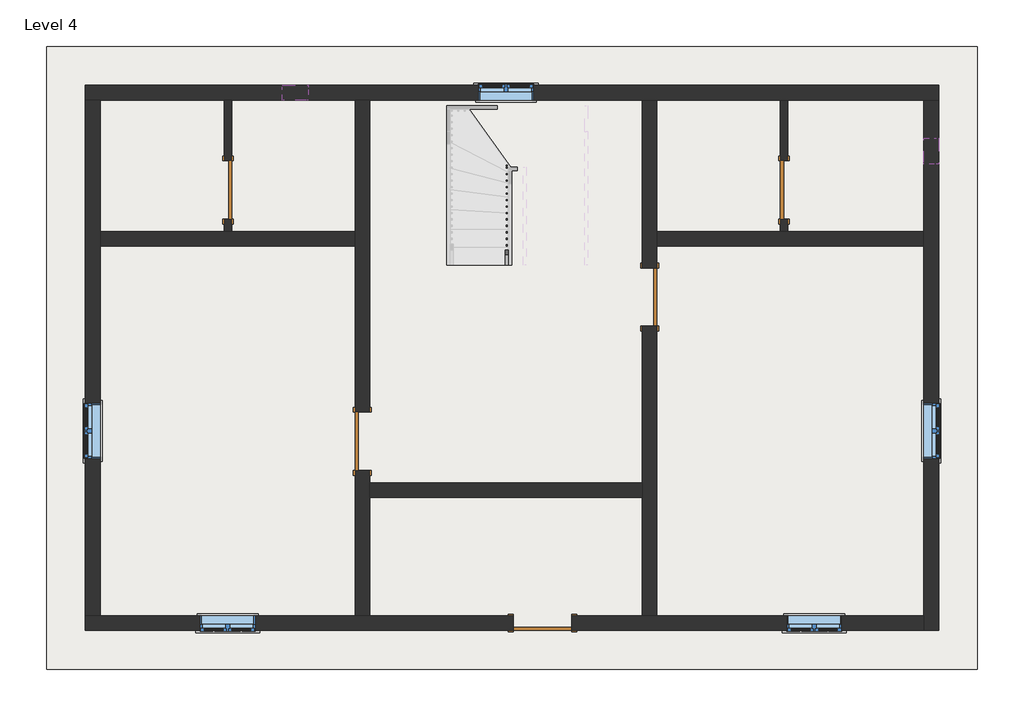
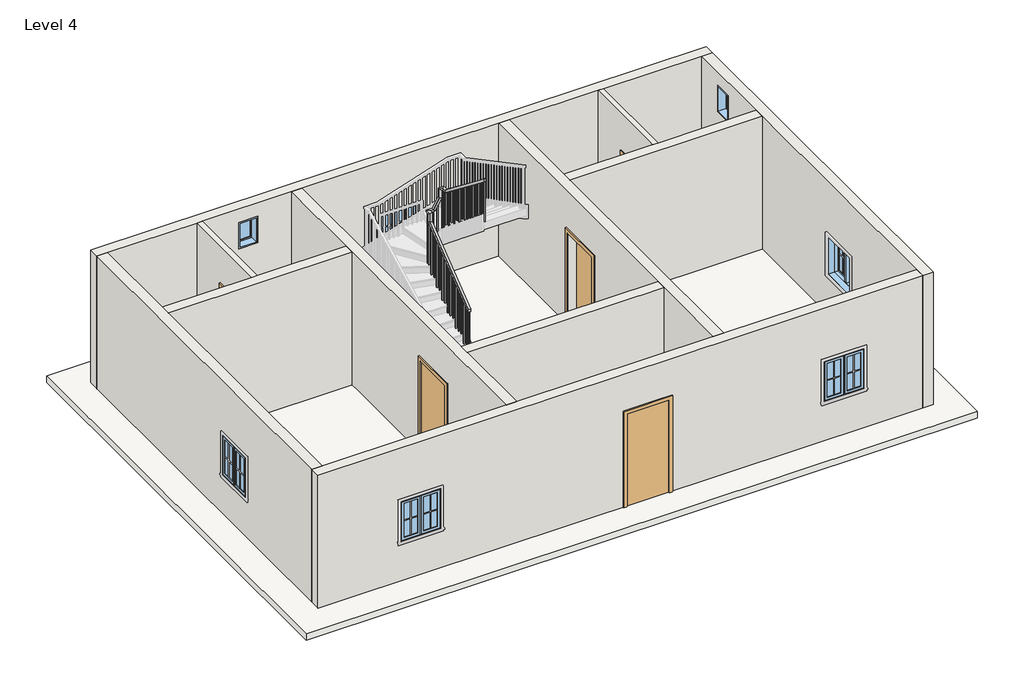
# One storey, part 1 of 2: 11 walls, 7 windows, 5 doors, 1 railing, 1 roof.
"""IFC4 building model written with IfcOpenShell, lengths in millimetres."""

from ifc_helpers import new_model, si_unit, frame, origin, place, context, project, spatial, polyline, outline, extrude, faceted_brep, transform, mapped, element, save
from components import door_e5f9f3c4, door_a90ba1ad, door_305aa2a5, door_0ca8825f, window_aa618e30, window_339605e1

model = new_model("IFC4")

# Units and contexts
model_context = context("Model", 3, world=origin())
ifc_project = project(units=[si_unit("LENGTHUNIT", "METRE", prefix="MILLI")], contexts=[model_context])

# Site, building, storey
site = spatial("IfcSite", under=ifc_project)
building = spatial("IfcBuilding", under=site)
storey = spatial("IfcBuildingStorey", under=building, Name="Level 4", Elevation=6400.8)

# Doors
placement = place(None, origin())
door_shape = door_e5f9f3c4(model_context)
element("IfcDoor", 1, ObjectType="Single-Flush : 36\" x 84\"", at=placement, inside=storey, context=model_context, shape_type="MappedRepresentation", body=[
    mapped(door_shape, transform((-5102.9390964, 4820.103532, 6400.8), x_axis=(0.0, -1.0, 0.0), y_axis=(1.0, 0.0, 0.0), z_axis=(0.0, 0.0, 1.0))),
])
door_2_shape = door_a90ba1ad(model_context)
element("IfcDoor", 2, ObjectType="Single-Flush : 36\" x 84\"", at=placement, inside=storey, context=model_context, shape_type="MappedRepresentation", body=[
    mapped(door_2_shape, transform((-3001.0890964, 883.103532, 6400.8), x_axis=(0.0, -1.0, 0.0), y_axis=(1.0, 0.0, 0.0), z_axis=(0.0, 0.0, 1.0))),
])
element("IfcDoor", 3, ObjectType="Single-Flush : 36\" x 84\"", at=placement, inside=storey, context=model_context, shape_type="MappedRepresentation", body=[
    mapped(door_2_shape, transform((1494.7109036, 3143.703532, 6400.8), x_axis=(0.0, 1.0, 0.0), y_axis=(-1.0, 0.0, 0.0), z_axis=(0.0, 0.0, 1.0))),
])
door_3_shape = door_305aa2a5(model_context)
element("IfcDoor", 4, ObjectType="Single-Flush : 36\" x 84\"", at=placement, inside=storey, context=model_context, shape_type="MappedRepresentation", body=[
    mapped(door_3_shape, transform((3596.5609036, 4820.103532, 6400.8), x_axis=(0.0, -1.0, 0.0), y_axis=(1.0, 0.0, 0.0), z_axis=(0.0, 0.0, 1.0))),
])
door_4_shape = door_0ca8825f(model_context)
element("IfcDoor", 5, ObjectType="Single-Flush : 36\" x 84\"", at=placement, inside=storey, context=model_context, shape_type="MappedRepresentation", body=[
    mapped(door_4_shape, transform((-181.6890964, -1961.696468, 6400.8), x_axis=(-1.0, 0.0, 0.0), y_axis=(0.0, -1.0, 0.0), z_axis=(0.0, 0.0, 1.0))),
])

# Railing
element("IfcRailing", 6, ObjectType="Handrail - Rectangular", at=placement, inside=storey, context=model_context, shape_type="SolidModel", body=[
    faceted_brep([(-765.8890964, 3647.9718401, 7484.5333333), (-765.8890964, 3647.9718401, 7420.2000346), (-715.0890964, 3647.9718401, 7420.2000346), (-715.0890964, 3647.9718401, 7484.5333333), (-765.8890964, 5099.503532, 8612.4191036), (-765.8890964, 5150.303532, 8587.5590024), (-715.0890964, 5150.303532, 8587.5590024), (-715.0890964, 5099.503532, 8612.4191036), (-765.8890964, 5099.503532, 8815.4281882), (-765.8890964, 5150.303532, 8764.6281882), (-715.0890964, 5150.303532, 8764.6281882), (-715.0890964, 5099.503532, 8815.4281882), (-765.8890964, 5226.503532, 8815.4281882), (-765.8890964, 5226.503532, 8764.6281882), (-715.0890964, 5175.703532, 8764.6281882), (-715.0890964, 5175.703532, 8815.4281882), (-638.8890964, 5226.503532, 8815.4281882), (-609.7677625, 5226.503532, 8764.6281882), (-609.7677625, 5175.703532, 8764.6281882), (-638.8890964, 5175.703532, 8815.4281882), (-511.8890964, 5226.503532, 9032.3051451), (-461.0890964, 5226.503532, 9018.5256424), (-461.0890964, 5175.703532, 9018.5256424), (-511.8890964, 5175.703532, 9032.3051451), (-511.8890964, 5226.503532, 9235.3142297), (-461.0890964, 5226.503532, 9184.5142297), (-461.0890964, 5175.703532, 9184.5142297), (-511.8890964, 5175.703532, 9235.3142297), (-384.8890964, 5226.503532, 9235.3142297), (-384.8890964, 5226.503532, 9184.5142297), (-435.6890964, 5175.703532, 9184.5142297), (-435.6890964, 5175.703532, 9235.3142297), (-384.8890964, 5099.503532, 9235.3142297), (-384.8890964, 5082.086864, 9184.5142297), (-435.6890964, 5082.086864, 9184.5142297), (-435.6890964, 5099.503532, 9235.3142297), (-384.8890964, 3647.9718401, 10363.2), (-435.6890964, 3647.9718401, 10363.2), (-435.6890964, 3647.9718401, 10298.8667013), (-384.8890964, 3647.9718401, 10298.8667013)], [[[0, 1, 2, 3]], [[1, 0, 4, 5]], [[2, 1, 5, 6]], [[3, 2, 6, 7]], [[0, 3, 7, 4]], [[5, 4, 8, 9]], [[6, 5, 9, 10]], [[7, 6, 10, 11]], [[4, 7, 11, 8]], [[9, 8, 12, 13]], [[10, 9, 13, 14]], [[11, 10, 14, 15]], [[8, 11, 15, 12]], [[13, 12, 16, 17]], [[14, 13, 17, 18]], [[15, 14, 18, 19]], [[12, 15, 19, 16]], [[17, 16, 20, 21]], [[18, 17, 21, 22]], [[19, 18, 22, 23]], [[16, 19, 23, 20]], [[21, 20, 24, 25]], [[22, 21, 25, 26]], [[23, 22, 26, 27]], [[20, 23, 27, 24]], [[25, 24, 28, 29]], [[26, 25, 29, 30]], [[27, 26, 30, 31]], [[24, 27, 31, 28]], [[29, 28, 32, 33]], [[30, 29, 33, 34]], [[31, 30, 34, 35]], [[28, 31, 35, 32]], [[36, 37, 38, 39]], [[33, 32, 36, 39]], [[34, 33, 39, 38]], [[35, 34, 38, 37]], [[32, 35, 37, 36]]]),
    extrude(outline(polyline([(3667.578532, 10283.6316852), (3686.628532, 10268.8292361), (3686.628532, 9279.4666667), (3667.578532, 9279.4666667), (3667.578532, 10283.6316852)])), frame((-419.8140964, 0.0, 0.0), z_axis=(1.0, 0.0, 0.0), x_axis=(0.0, 1.0, 0.0)), (0.0, 0.0, 1.0), 19.05),
    extrude(outline(polyline([(3769.178532, 10204.6852902), (3788.228532, 10189.8828411), (3788.228532, 9279.4666667), (3769.178532, 9279.4666667), (3769.178532, 10204.6852902)])), frame((-419.8140964, 0.0, 0.0), z_axis=(1.0, 0.0, 0.0), x_axis=(0.0, 1.0, 0.0)), (0.0, 0.0, 1.0), 19.05),
    extrude(outline(polyline([(3870.778532, 10125.7388952), (3889.828532, 10110.9364462), (3889.828532, 9279.4666667), (3870.778532, 9279.4666667), (3870.778532, 10125.7388952)])), frame((-419.8140964, 0.0, 0.0), z_axis=(1.0, 0.0, 0.0), x_axis=(0.0, 1.0, 0.0)), (0.0, 0.0, 1.0), 19.05),
    extrude(outline(polyline([(3972.378532, 10046.7925003), (3991.428532, 10031.9900512), (3991.428532, 9110.1333333), (3972.378532, 9110.1333333), (3972.378532, 10046.7925003)])), frame((-419.8140964, 0.0, 0.0), z_axis=(1.0, 0.0, 0.0), x_axis=(0.0, 1.0, 0.0)), (0.0, 0.0, 1.0), 19.05),
    extrude(outline(polyline([(4073.978532, 9967.8461053), (4093.028532, 9953.0436562), (4093.028532, 9110.1333333), (4073.978532, 9110.1333333), (4073.978532, 9967.8461053)])), frame((-419.8140964, 0.0, 0.0), z_axis=(1.0, 0.0, 0.0), x_axis=(0.0, 1.0, 0.0)), (0.0, 0.0, 1.0), 19.05),
    extrude(outline(polyline([(4175.578532, 9888.8997103), (4194.628532, 9874.0972613), (4194.628532, 9110.1333333), (4175.578532, 9110.1333333), (4175.578532, 9888.8997103)])), frame((-419.8140964, 0.0, 0.0), z_axis=(1.0, 0.0, 0.0), x_axis=(0.0, 1.0, 0.0)), (0.0, 0.0, 1.0), 19.05),
    extrude(outline(polyline([(4277.178532, 9809.9533154), (4296.228532, 9795.1508663), (4296.228532, 8940.8), (4277.178532, 8940.8), (4277.178532, 9809.9533154)])), frame((-419.8140964, 0.0, 0.0), z_axis=(1.0, 0.0, 0.0), x_axis=(0.0, 1.0, 0.0)), (0.0, 0.0, 1.0), 19.05),
    extrude(outline(polyline([(4378.778532, 9731.0069204), (4397.828532, 9716.2044713), (4397.828532, 8940.8), (4378.778532, 8940.8), (4378.778532, 9731.0069204)])), frame((-419.8140964, 0.0, 0.0), z_axis=(1.0, 0.0, 0.0), x_axis=(0.0, 1.0, 0.0)), (0.0, 0.0, 1.0), 19.05),
    extrude(outline(polyline([(4480.378532, 9652.0605254), (4499.428532, 9637.2580764), (4499.428532, 8771.4666667), (4480.378532, 8771.4666667), (4480.378532, 9652.0605254)])), frame((-419.8140964, 0.0, 0.0), z_axis=(1.0, 0.0, 0.0), x_axis=(0.0, 1.0, 0.0)), (0.0, 0.0, 1.0), 19.05),
    extrude(outline(polyline([(4581.978532, 9573.1141304), (4601.028532, 9558.3116814), (4601.028532, 8771.4666667), (4581.978532, 8771.4666667), (4581.978532, 9573.1141304)])), frame((-419.8140964, 0.0, 0.0), z_axis=(1.0, 0.0, 0.0), x_axis=(0.0, 1.0, 0.0)), (0.0, 0.0, 1.0), 19.05),
    extrude(outline(polyline([(4683.578532, 9494.1677355), (4702.628532, 9479.3652864), (4702.628532, 8771.4666667), (4683.578532, 8771.4666667), (4683.578532, 9494.1677355)])), frame((-419.8140964, 0.0, 0.0), z_axis=(1.0, 0.0, 0.0), x_axis=(0.0, 1.0, 0.0)), (0.0, 0.0, 1.0), 19.05),
    extrude(outline(polyline([(4785.178532, 9415.2213405), (4804.228532, 9400.4188914), (4804.228532, 8602.1333333), (4785.178532, 8602.1333333), (4785.178532, 9415.2213405)])), frame((-419.8140964, 0.0, 0.0), z_axis=(1.0, 0.0, 0.0), x_axis=(0.0, 1.0, 0.0)), (0.0, 0.0, 1.0), 19.05),
    extrude(outline(polyline([(4886.778532, 9336.2749455), (4905.828532, 9321.4724965), (4905.828532, 8602.1333333), (4886.778532, 8602.1333333), (4886.778532, 9336.2749455)])), frame((-419.8140964, 0.0, 0.0), z_axis=(1.0, 0.0, 0.0), x_axis=(0.0, 1.0, 0.0)), (0.0, 0.0, 1.0), 19.05),
    extrude(outline(polyline([(4988.378532, 9257.3285506), (5007.428532, 9242.5261015), (5007.428532, 8432.8), (4988.378532, 8432.8), (4988.378532, 9257.3285506)])), frame((-419.8140964, 0.0, 0.0), z_axis=(1.0, 0.0, 0.0), x_axis=(0.0, 1.0, 0.0)), (0.0, 0.0, 1.0), 19.05),
    extrude(outline(polyline([(5089.978532, 9178.3821556), (5109.028532, 9163.5797065), (5109.028532, 8432.8), (5089.978532, 8432.8), (5089.978532, 9178.3821556)])), frame((-419.8140964, 0.0, 0.0), z_axis=(1.0, 0.0, 0.0), x_axis=(0.0, 1.0, 0.0)), (0.0, 0.0, 1.0), 19.05),
    extrude(outline(polyline([(-445.2140964, 5191.578532), (-445.2140964, 5210.628532), (-426.1640964, 5210.628532), (-426.1640964, 5191.578532), (-445.2140964, 5191.578532)])), frame((0.0, 0.0, 8094.1333333), z_axis=(0.0, 0.0, 1.0), x_axis=(1.0, 0.0, 0.0)), (0.0, 0.0, 1.0), 1090.3808964),
    extrude(outline(polyline([(8904.66524, -527.7640964), (8872.1336964, -546.8140964), (7924.8, -546.8140964), (7924.8, -527.7640964), (8904.66524, -527.7640964)])), frame((0.0, 5191.578532, 0.0), z_axis=(0.0, 1.0, 0.0), x_axis=(0.0, 0.0, 1.0)), (0.0, 0.0, 1.0), 19.05),
    extrude(outline(polyline([(8731.1636744, -629.3640964), (8698.6321309, -648.4140964), (7755.4666667, -648.4140964), (7755.4666667, -629.3640964), (8731.1636744, -629.3640964)])), frame((0.0, 5191.578532, 0.0), z_axis=(0.0, 1.0, 0.0), x_axis=(0.0, 0.0, 1.0)), (0.0, 0.0, 1.0), 19.05),
    extrude(outline(polyline([(-730.9640964, 5162.4468401), (-750.0140964, 5162.4468401), (-750.0140964, 5181.4968401), (-730.9640964, 5181.4968401), (-730.9640964, 5162.4468401)])), frame((0.0, 0.0, 7586.1333333), z_axis=(0.0, 0.0, 1.0), x_axis=(1.0, 0.0, 0.0)), (0.0, 0.0, 1.0), 1178.4948549),
    extrude(outline(polyline([(5060.8468401, 8518.0483397), (5079.8968401, 8532.8507888), (5079.8968401, 7416.8), (5060.8468401, 7416.8), (5060.8468401, 8518.0483397)])), frame((-750.0140964, 0.0, 0.0), z_axis=(1.0, 0.0, 0.0), x_axis=(0.0, 1.0, 0.0)), (0.0, 0.0, 1.0), 19.05),
    extrude(outline(polyline([(4959.2468401, 8439.1019447), (4978.2968401, 8453.9043938), (4978.2968401, 7416.8), (4959.2468401, 7416.8), (4959.2468401, 8439.1019447)])), frame((-750.0140964, 0.0, 0.0), z_axis=(1.0, 0.0, 0.0), x_axis=(0.0, 1.0, 0.0)), (0.0, 0.0, 1.0), 19.05),
    extrude(outline(polyline([(4857.6468401, 8360.1555498), (4876.6968401, 8374.9579988), (4876.6968401, 7247.4666667), (4857.6468401, 7247.4666667), (4857.6468401, 8360.1555498)])), frame((-750.0140964, 0.0, 0.0), z_axis=(1.0, 0.0, 0.0), x_axis=(0.0, 1.0, 0.0)), (0.0, 0.0, 1.0), 19.05),
    extrude(outline(polyline([(4756.0468401, 8281.2091548), (4775.0968401, 8296.0116039), (4775.0968401, 7247.4666667), (4756.0468401, 7247.4666667), (4756.0468401, 8281.2091548)])), frame((-750.0140964, 0.0, 0.0), z_axis=(1.0, 0.0, 0.0), x_axis=(0.0, 1.0, 0.0)), (0.0, 0.0, 1.0), 19.05),
    extrude(outline(polyline([(4654.4468401, 8202.2627598), (4673.4968401, 8217.0652089), (4673.4968401, 7078.1333333), (4654.4468401, 7078.1333333), (4654.4468401, 8202.2627598)])), frame((-750.0140964, 0.0, 0.0), z_axis=(1.0, 0.0, 0.0), x_axis=(0.0, 1.0, 0.0)), (0.0, 0.0, 1.0), 19.05),
    extrude(outline(polyline([(4552.8468401, 8123.3163649), (4571.8968401, 8138.1188139), (4571.8968401, 7078.1333333), (4552.8468401, 7078.1333333), (4552.8468401, 8123.3163649)])), frame((-750.0140964, 0.0, 0.0), z_axis=(1.0, 0.0, 0.0), x_axis=(0.0, 1.0, 0.0)), (0.0, 0.0, 1.0), 19.05),
    extrude(outline(polyline([(4451.2468401, 8044.3699699), (4470.2968401, 8059.1724189), (4470.2968401, 6908.8), (4451.2468401, 6908.8), (4451.2468401, 8044.3699699)])), frame((-750.0140964, 0.0, 0.0), z_axis=(1.0, 0.0, 0.0), x_axis=(0.0, 1.0, 0.0)), (0.0, 0.0, 1.0), 19.05),
    extrude(outline(polyline([(4349.6468401, 7965.4235749), (4368.6968401, 7980.226024), (4368.6968401, 6908.8), (4349.6468401, 6908.8), (4349.6468401, 7965.4235749)])), frame((-750.0140964, 0.0, 0.0), z_axis=(1.0, 0.0, 0.0), x_axis=(0.0, 1.0, 0.0)), (0.0, 0.0, 1.0), 19.05),
    extrude(outline(polyline([(4248.0468401, 7886.4771799), (4267.0968401, 7901.279629), (4267.0968401, 6908.8), (4248.0468401, 6908.8), (4248.0468401, 7886.4771799)])), frame((-750.0140964, 0.0, 0.0), z_axis=(1.0, 0.0, 0.0), x_axis=(0.0, 1.0, 0.0)), (0.0, 0.0, 1.0), 19.05),
    extrude(outline(polyline([(4146.4468401, 7807.530785), (4165.4968401, 7822.333234), (4165.4968401, 6739.4666667), (4146.4468401, 6739.4666667), (4146.4468401, 7807.530785)])), frame((-750.0140964, 0.0, 0.0), z_axis=(1.0, 0.0, 0.0), x_axis=(0.0, 1.0, 0.0)), (0.0, 0.0, 1.0), 19.05),
    extrude(outline(polyline([(4044.8468401, 7728.58439), (4063.8968401, 7743.3868391), (4063.8968401, 6739.4666667), (4044.8468401, 6739.4666667), (4044.8468401, 7728.58439)])), frame((-750.0140964, 0.0, 0.0), z_axis=(1.0, 0.0, 0.0), x_axis=(0.0, 1.0, 0.0)), (0.0, 0.0, 1.0), 19.05),
    extrude(outline(polyline([(3943.2468401, 7649.637995), (3962.2968401, 7664.4404441), (3962.2968401, 6739.4666667), (3943.2468401, 6739.4666667), (3943.2468401, 7649.637995)])), frame((-750.0140964, 0.0, 0.0), z_axis=(1.0, 0.0, 0.0), x_axis=(0.0, 1.0, 0.0)), (0.0, 0.0, 1.0), 19.05),
    extrude(outline(polyline([(3841.6468401, 7570.6916001), (3860.6968401, 7585.4940491), (3860.6968401, 6570.1333333), (3841.6468401, 6570.1333333), (3841.6468401, 7570.6916001)])), frame((-750.0140964, 0.0, 0.0), z_axis=(1.0, 0.0, 0.0), x_axis=(0.0, 1.0, 0.0)), (0.0, 0.0, 1.0), 19.05),
    extrude(outline(polyline([(3740.0468401, 7491.7452051), (3759.0968401, 7506.5476541), (3759.0968401, 6570.1333333), (3740.0468401, 6570.1333333), (3740.0468401, 7491.7452051)])), frame((-750.0140964, 0.0, 0.0), z_axis=(1.0, 0.0, 0.0), x_axis=(0.0, 1.0, 0.0)), (0.0, 0.0, 1.0), 19.05),
    extrude(outline(polyline([(-419.8140964, 5191.578532), (-419.8140964, 5210.628532), (-400.7640964, 5210.628532), (-400.7640964, 5191.578532), (-419.8140964, 5191.578532)])), frame((0.0, 0.0, 8263.4666667), z_axis=(0.0, 0.0, 1.0), x_axis=(1.0, 0.0, 0.0)), (0.0, 0.0, 1.0), 921.0475631),
    extrude(outline(polyline([(-730.9640964, 5191.578532), (-750.0140964, 5191.578532), (-750.0140964, 5210.628532), (-730.9640964, 5210.628532), (-730.9640964, 5191.578532)])), frame((0.0, 0.0, 7586.1333333), z_axis=(0.0, 0.0, 1.0), x_axis=(1.0, 0.0, 0.0)), (0.0, 0.0, 1.0), 1178.4948549),
    extrude(outline(polyline([(3647.9718401, 10298.8667013), (3667.0218401, 10284.0642523), (3667.0218401, 9279.4666667), (3647.9718401, 9279.4666667), (3647.9718401, 10298.8667013)])), frame((-419.8140964, 0.0, 0.0), z_axis=(1.0, 0.0, 0.0), x_axis=(0.0, 1.0, 0.0)), (0.0, 0.0, 1.0), 19.05),
    extrude(outline(polyline([(3647.9718401, 7420.2000346), (3667.0218401, 7435.0024837), (3667.0218401, 6570.1333333), (3647.9718401, 6570.1333333), (3647.9718401, 7420.2000346)])), frame((-750.0140964, 0.0, 0.0), z_axis=(1.0, 0.0, 0.0), x_axis=(0.0, 1.0, 0.0)), (0.0, 0.0, 1.0), 19.05),
])

# Roof
element("IfcRoof", 7, ObjectType="Generic - 12\"", at=placement, inside=storey, context=model_context, shape_type="SweptSolid", body=[
    extrude(outline(polyline([(-7944.5640964, 7068.003532), (6625.5109036, 7068.003532), (6625.5109036, -2685.596468), (-7944.5640964, -2685.596468), (-7944.5640964, 7068.003532)])), frame((0.0, 0.0, 6248.4), z_axis=(0.0, 0.0, 1.0), x_axis=(1.0, 0.0, 0.0)), (0.0, 0.0, 1.0), 152.4),
])

# Walls
element("IfcWall", 8, ObjectType="WALL4.5\"", at=placement, inside=storey, context=model_context, shape_type="SweptSolid", body=[
    extrude(outline(polyline([(4362.903532, 8534.4), (4362.903532, 6400.8), (4172.403532, 6400.8), (4172.403532, 9448.8), (6229.803532, 9448.8), (6229.803532, 6400.8), (5277.303532, 6400.8), (5277.303532, 8534.4), (4362.903532, 8534.4)])), frame((-5160.0890964, 0.0, 0.0), z_axis=(1.0, 0.0, 0.0), x_axis=(0.0, 1.0, 0.0)), (0.0, 0.0, 1.0), 114.3),
])
element("IfcWall", 9, ObjectType="WALL4.5\"", at=placement, inside=storey, context=model_context, shape_type="SweptSolid", body=[
    extrude(outline(polyline([(4362.903532, 8534.4), (4362.903532, 6400.8), (4172.403532, 6400.8), (4172.403532, 9448.8), (6229.803532, 9448.8), (6229.803532, 6400.8), (5277.303532, 6400.8), (5277.303532, 8534.4), (4362.903532, 8534.4)])), frame((3539.4109036, 0.0, 0.0), z_axis=(1.0, 0.0, 0.0), x_axis=(0.0, 1.0, 0.0)), (0.0, 0.0, 1.0), 114.3),
])
element("IfcWall", 10, ObjectType="WALL9\"", at=placement, inside=storey, context=model_context, shape_type="Brep", body=[
    faceted_brep([(-7334.9640964, 6229.803532, 6400.8), (-7106.3640964, 6229.803532, 6400.8), (-5160.0890964, 6229.803532, 6400.8), (-5045.7890964, 6229.803532, 6400.8), (-3115.3890964, 6229.803532, 6400.8), (-2886.7890964, 6229.803532, 6400.8), (1380.4109036, 6229.803532, 6400.8), (1609.0109036, 6229.803532, 6400.8), (3539.4109036, 6229.803532, 6400.8), (3653.7109036, 6229.803532, 6400.8), (5787.3109036, 6229.803532, 6400.8), (6015.9109036, 6229.803532, 6400.8), (6015.9109036, 6229.803532, 9448.8), (5787.3109036, 6229.803532, 9448.8), (3653.7109036, 6229.803532, 9448.8), (3539.4109036, 6229.803532, 9448.8), (1609.0109036, 6229.803532, 9448.8), (1380.4109036, 6229.803532, 9448.8), (-2886.7890964, 6229.803532, 9448.8), (-3115.3890964, 6229.803532, 9448.8), (-5045.7890964, 6229.803532, 9448.8), (-5160.0890964, 6229.803532, 9448.8), (-7106.3640964, 6229.803532, 9448.8), (-7334.9640964, 6229.803532, 9448.8), (-3848.8140964, 6229.803532, 9144.0), (-3848.8140964, 6229.803532, 8534.4), (-4255.2140964, 6229.803532, 8534.4), (-4255.2140964, 6229.803532, 9144.0), (-321.3890964, 6229.803532, 8229.6), (-321.3890964, 6229.803532, 7315.2), (-1184.9890964, 6229.803532, 7315.2), (-1184.9890964, 6229.803532, 8229.6), (-7334.9640964, 6458.403532, 6400.8), (-7334.9640964, 6458.403532, 9448.8), (6015.9109036, 6458.403532, 9448.8), (6015.9109036, 6458.403532, 6400.8), (-3848.8140964, 6458.403532, 9144.0), (-4255.2140964, 6458.403532, 9144.0), (-4255.2140964, 6458.403532, 8534.4), (-3848.8140964, 6458.403532, 8534.4), (-321.3890964, 6458.403532, 8229.6), (-1184.9890964, 6458.403532, 8229.6), (-1184.9890964, 6458.403532, 7315.2), (-321.3890964, 6458.403532, 7315.2)], [[[0, 1, 2, 3, 4, 5, 6, 7, 8, 9, 10, 11, 12, 13, 14, 15, 16, 17, 18, 19, 20, 21, 22, 23], [24, 25, 26, 27], [28, 29, 30, 31]], [[32, 33, 34, 35], [36, 37, 38, 39], [40, 41, 42, 43]], [[11, 10, 9, 8, 7, 6, 5, 4, 3, 2, 1, 0, 32, 35]], [[12, 11, 35, 34]], [[0, 23, 33, 32]], [[25, 24, 36, 39]], [[26, 25, 39, 38]], [[27, 26, 38, 37]], [[24, 27, 37, 36]], [[29, 28, 40, 43]], [[30, 29, 43, 42]], [[31, 30, 42, 41]], [[28, 31, 41, 40]], [[23, 22, 21, 20, 19, 18, 17, 16, 15, 14, 13, 12, 34, 33]]]),
])
element("IfcWall", 11, ObjectType="WALL9\"", at=placement, inside=storey, context=model_context, shape_type="Brep", body=[
    faceted_brep([(5787.3109036, 6229.803532, 6400.8), (5787.3109036, 4172.403532, 6400.8), (5787.3109036, 3943.803532, 6400.8), (5787.3109036, -1847.396468, 6400.8), (5787.3109036, -2075.996468, 6400.8), (5787.3109036, -2075.996468, 9448.8), (5787.3109036, -1847.396468, 9448.8), (5787.3109036, 3943.803532, 9448.8), (5787.3109036, 4172.403532, 9448.8), (5787.3109036, 6229.803532, 9448.8), (5787.3109036, 5226.503532, 9144.0), (5787.3109036, 5226.503532, 8534.4), (5787.3109036, 5632.903532, 8534.4), (5787.3109036, 5632.903532, 9144.0), (5787.3109036, 616.403532, 8229.6), (5787.3109036, 616.403532, 7315.2), (5787.3109036, 1480.003532, 7315.2), (5787.3109036, 1480.003532, 8229.6), (6015.9109036, 6229.803532, 6400.8), (6015.9109036, 6229.803532, 9448.8), (6015.9109036, -2075.996468, 9448.8), (6015.9109036, -2075.996468, 6400.8), (6015.9109036, 5226.503532, 9144.0), (6015.9109036, 5632.903532, 9144.0), (6015.9109036, 5632.903532, 8534.4), (6015.9109036, 5226.503532, 8534.4), (6015.9109036, 616.403532, 8229.6), (6015.9109036, 1480.003532, 8229.6), (6015.9109036, 1480.003532, 7315.2), (6015.9109036, 616.403532, 7315.2)], [[[0, 1, 2, 3, 4, 5, 6, 7, 8, 9], [10, 11, 12, 13], [14, 15, 16, 17]], [[18, 19, 20, 21], [22, 23, 24, 25], [26, 27, 28, 29]], [[4, 3, 2, 1, 0, 18, 21]], [[0, 9, 19, 18]], [[5, 4, 21, 20]], [[11, 10, 22, 25]], [[12, 11, 25, 24]], [[13, 12, 24, 23]], [[10, 13, 23, 22]], [[15, 14, 26, 29]], [[16, 15, 29, 28]], [[17, 16, 28, 27]], [[14, 17, 27, 26]], [[9, 8, 7, 6, 5, 20, 19]]]),
])
element("IfcWall", 12, ObjectType="WALL9\"", at=placement, inside=storey, context=model_context, shape_type="Brep", body=[
    faceted_brep([(-638.8890964, -1847.396468, 8534.4), (-638.8890964, -1847.396468, 6400.8), (-2886.7890964, -1847.396468, 6400.8), (-3115.3890964, -1847.396468, 6400.8), (-7106.3640964, -1847.396468, 6400.8), (-7334.9640964, -1847.396468, 6400.8), (-7334.9640964, -1847.396468, 9448.8), (-7106.3640964, -1847.396468, 9448.8), (-3115.3890964, -1847.396468, 9448.8), (-2886.7890964, -1847.396468, 9448.8), (1380.4109036, -1847.396468, 9448.8), (1609.0109036, -1847.396468, 9448.8), (5787.3109036, -1847.396468, 9448.8), (5787.3109036, -1847.396468, 6400.8), (1609.0109036, -1847.396468, 6400.8), (1380.4109036, -1847.396468, 6400.8), (275.5109036, -1847.396468, 6400.8), (275.5109036, -1847.396468, 8534.4), (-5542.6765964, -1847.396468, 8229.6), (-5542.6765964, -1847.396468, 7315.2), (-4679.0765964, -1847.396468, 7315.2), (-4679.0765964, -1847.396468, 8229.6), (3641.0109036, -1847.396468, 8229.6), (3641.0109036, -1847.396468, 7315.2), (4504.6109036, -1847.396468, 7315.2), (4504.6109036, -1847.396468, 8229.6), (-7334.9640964, -2075.996468, 6400.8), (-638.8890964, -2075.996468, 6400.8), (-638.8890964, -2075.996468, 8534.4), (275.5109036, -2075.996468, 8534.4), (275.5109036, -2075.996468, 6400.8), (5787.3109036, -2075.996468, 6400.8), (5787.3109036, -2075.996468, 9448.8), (-7334.9640964, -2075.996468, 9448.8), (-5542.6765964, -2075.996468, 8229.6), (-4679.0765964, -2075.996468, 8229.6), (-4679.0765964, -2075.996468, 7315.2), (-5542.6765964, -2075.996468, 7315.2), (3641.0109036, -2075.996468, 8229.6), (4504.6109036, -2075.996468, 8229.6), (4504.6109036, -2075.996468, 7315.2), (3641.0109036, -2075.996468, 7315.2)], [[[0, 1, 2, 3, 4, 5, 6, 7, 8, 9, 10, 11, 12, 13, 14, 15, 16, 17], [18, 19, 20, 21], [22, 23, 24, 25]], [[26, 27, 28, 29, 30, 31, 32, 33], [34, 35, 36, 37], [38, 39, 40, 41]], [[5, 4, 3, 2, 1, 27, 26]], [[16, 15, 14, 13, 31, 30]], [[13, 12, 32, 31]], [[6, 5, 26, 33]], [[19, 18, 34, 37]], [[20, 19, 37, 36]], [[21, 20, 36, 35]], [[18, 21, 35, 34]], [[23, 22, 38, 41]], [[24, 23, 41, 40]], [[25, 24, 40, 39]], [[22, 25, 39, 38]], [[12, 11, 10, 9, 8, 7, 6, 33, 32]], [[28, 27, 1, 0]], [[29, 28, 0, 17]], [[30, 29, 17, 16]]]),
])
element("IfcWall", 13, ObjectType="WALL9\"", at=placement, inside=storey, context=model_context, shape_type="Brep", body=[
    faceted_brep([(-7106.3640964, -1847.396468, 6400.8), (-7106.3640964, 3943.803532, 6400.8), (-7106.3640964, 4172.403532, 6400.8), (-7106.3640964, 6229.803532, 6400.8), (-7106.3640964, 6229.803532, 9448.8), (-7106.3640964, 4172.403532, 9448.8), (-7106.3640964, 3943.803532, 9448.8), (-7106.3640964, -1847.396468, 9448.8), (-7106.3640964, 1480.003532, 8229.6), (-7106.3640964, 1480.003532, 7315.2), (-7106.3640964, 616.403532, 7315.2), (-7106.3640964, 616.403532, 8229.6), (-7334.9640964, -1847.396468, 6400.8), (-7334.9640964, -1847.396468, 9448.8), (-7334.9640964, 6229.803532, 9448.8), (-7334.9640964, 6229.803532, 6400.8), (-7334.9640964, 1480.003532, 8229.6), (-7334.9640964, 616.403532, 8229.6), (-7334.9640964, 616.403532, 7315.2), (-7334.9640964, 1480.003532, 7315.2)], [[[0, 1, 2, 3, 4, 5, 6, 7], [8, 9, 10, 11]], [[12, 13, 14, 15], [16, 17, 18, 19]], [[3, 2, 1, 0, 12, 15]], [[0, 7, 13, 12]], [[4, 3, 15, 14]], [[9, 8, 16, 19]], [[10, 9, 19, 18]], [[11, 10, 18, 17]], [[8, 11, 17, 16]], [[7, 6, 5, 4, 14, 13]]]),
])
element("IfcWall", 14, ObjectType="WALL9\"", at=placement, inside=storey, context=model_context, shape_type="Brep", body=[
    faceted_brep([(-3115.3890964, 425.903532, 8534.4), (-3115.3890964, 425.903532, 6400.8), (-3115.3890964, -1847.396468, 6400.8), (-3115.3890964, -1847.396468, 9448.8), (-3115.3890964, 3943.803532, 9448.8), (-3115.3890964, 4172.403532, 9448.8), (-3115.3890964, 6229.803532, 9448.8), (-3115.3890964, 6229.803532, 6400.8), (-3115.3890964, 4172.403532, 6400.8), (-3115.3890964, 3943.803532, 6400.8), (-3115.3890964, 1340.303532, 6400.8), (-3115.3890964, 1340.303532, 8534.4), (-2886.7890964, -1847.396468, 6400.8), (-2886.7890964, 6.803532, 6400.8), (-2886.7890964, 235.403532, 6400.8), (-2886.7890964, 425.903532, 6400.8), (-2886.7890964, 425.903532, 8534.4), (-2886.7890964, 1340.303532, 8534.4), (-2886.7890964, 1340.303532, 6400.8), (-2886.7890964, 6229.803532, 6400.8), (-2886.7890964, 6229.803532, 9448.8), (-2886.7890964, 235.403532, 9448.8), (-2886.7890964, 6.803532, 9448.8), (-2886.7890964, -1847.396468, 9448.8)], [[[0, 1, 2, 3, 4, 5, 6, 7, 8, 9, 10, 11]], [[12, 13, 14, 15, 16, 17, 18, 19, 20, 21, 22, 23]], [[2, 1, 15, 14, 13, 12]], [[10, 9, 8, 7, 19, 18]], [[7, 6, 20, 19]], [[3, 2, 12, 23]], [[16, 15, 1, 0]], [[17, 16, 0, 11]], [[18, 17, 11, 10]], [[6, 5, 4, 3, 23, 22, 21, 20]]]),
])
element("IfcWall", 15, ObjectType="WALL9\"", at=placement, inside=storey, context=model_context, shape_type="SweptSolid", body=[
    extrude(outline(polyline([(1380.4109036, 6.803532), (-2886.7890964, 6.803532), (-2886.7890964, 235.403532), (1380.4109036, 235.403532), (1380.4109036, 6.803532)])), frame((0.0, 0.0, 6400.8), z_axis=(0.0, 0.0, 1.0), x_axis=(1.0, 0.0, 0.0)), (0.0, 0.0, 1.0), 3048.0),
])
element("IfcWall", 16, ObjectType="WALL9\"", at=placement, inside=storey, context=model_context, shape_type="Brep", body=[
    faceted_brep([(1609.0109036, 3600.903532, 8534.4), (1609.0109036, 3600.903532, 6400.8), (1609.0109036, 3943.803532, 6400.8), (1609.0109036, 4172.403532, 6400.8), (1609.0109036, 6229.803532, 6400.8), (1609.0109036, 6229.803532, 9448.8), (1609.0109036, 4172.403532, 9448.8), (1609.0109036, 3943.803532, 9448.8), (1609.0109036, -1847.396468, 9448.8), (1609.0109036, -1847.396468, 6400.8), (1609.0109036, 2686.503532, 6400.8), (1609.0109036, 2686.503532, 8534.4), (1380.4109036, 6229.803532, 6400.8), (1380.4109036, 3600.903532, 6400.8), (1380.4109036, 3600.903532, 8534.4), (1380.4109036, 2686.503532, 8534.4), (1380.4109036, 2686.503532, 6400.8), (1380.4109036, 235.403532, 6400.8), (1380.4109036, 6.803532, 6400.8), (1380.4109036, -1847.396468, 6400.8), (1380.4109036, -1847.396468, 9448.8), (1380.4109036, 6.803532, 9448.8), (1380.4109036, 235.403532, 9448.8), (1380.4109036, 6229.803532, 9448.8)], [[[0, 1, 2, 3, 4, 5, 6, 7, 8, 9, 10, 11]], [[12, 13, 14, 15, 16, 17, 18, 19, 20, 21, 22, 23]], [[10, 9, 19, 18, 17, 16]], [[4, 3, 2, 1, 13, 12]], [[5, 4, 12, 23]], [[9, 8, 20, 19]], [[14, 13, 1, 0]], [[15, 14, 0, 11]], [[16, 15, 11, 10]], [[8, 7, 6, 5, 23, 22, 21, 20]]]),
])
element("IfcWall", 17, ObjectType="WALL9\"", at=placement, inside=storey, context=model_context, shape_type="Brep", body=[
    faceted_brep([(1609.0109036, 3943.803532, 6400.8), (5787.3109036, 3943.803532, 6400.8), (5787.3109036, 3943.803532, 9448.8), (1609.0109036, 3943.803532, 9448.8), (1609.0109036, 4172.403532, 6400.8), (1609.0109036, 4172.403532, 9448.8), (3539.4109036, 4172.403532, 9448.8), (3653.7109036, 4172.403532, 9448.8), (5787.3109036, 4172.403532, 9448.8), (5787.3109036, 4172.403532, 6400.8), (3653.7109036, 4172.403532, 6400.8), (3539.4109036, 4172.403532, 6400.8)], [[[0, 1, 2, 3]], [[4, 5, 6, 7, 8, 9, 10, 11]], [[1, 0, 4, 11, 10, 9]], [[2, 1, 9, 8]], [[0, 3, 5, 4]], [[3, 2, 8, 7, 6, 5]]]),
])
element("IfcWall", 18, ObjectType="WALL9\"", at=placement, inside=storey, context=model_context, shape_type="Brep", body=[
    faceted_brep([(-7106.3640964, 3943.803532, 6400.8), (-3115.3890964, 3943.803532, 6400.8), (-3115.3890964, 3943.803532, 9448.8), (-7106.3640964, 3943.803532, 9448.8), (-7106.3640964, 4172.403532, 6400.8), (-7106.3640964, 4172.403532, 9448.8), (-5160.0890964, 4172.403532, 9448.8), (-5045.7890964, 4172.403532, 9448.8), (-3115.3890964, 4172.403532, 9448.8), (-3115.3890964, 4172.403532, 6400.8), (-5045.7890964, 4172.403532, 6400.8), (-5160.0890964, 4172.403532, 6400.8)], [[[0, 1, 2, 3]], [[4, 5, 6, 7, 8, 9, 10, 11]], [[1, 0, 4, 11, 10, 9]], [[0, 3, 5, 4]], [[2, 1, 9, 8]], [[3, 2, 8, 7, 6, 5]]]),
])

# Windows
window_shape = window_aa618e30(model_context)
element("IfcWindow", 19, ObjectType="Fixed : 16\" x 24\"", at=placement, inside=storey, context=model_context, shape_type="MappedRepresentation", body=[
    mapped(window_shape, transform((-4013.9140964, 6344.103532, 7620.0), x_axis=(1.0, 0.0, 0.0), y_axis=(0.0, 1.0, 0.0), z_axis=(0.0, 0.0, 1.0))),
])
element("IfcWindow", 20, ObjectType="Fixed : 16\" x 24\"", at=placement, inside=storey, context=model_context, shape_type="MappedRepresentation", body=[
    mapped(window_shape, transform((5901.6109036, 5391.603532, 7620.0), x_axis=(0.0, -1.0, 0.0), y_axis=(1.0, 0.0, 0.0), z_axis=(0.0, 0.0, 1.0))),
])
window_2_shape = window_339605e1(model_context)
element("IfcWindow", 21, ObjectType="Window-Casement-Double : 34\" x 36\"", at=placement, inside=storey, context=model_context, shape_type="MappedRepresentation", body=[
    mapped(window_2_shape, transform((-7220.6640964, 1048.203532, 6400.8), x_axis=(0.0, 1.0, 0.0), y_axis=(-1.0, 0.0, 0.0), z_axis=(0.0, 0.0, 1.0))),
])
element("IfcWindow", 22, ObjectType="Window-Casement-Double : 34\" x 36\"", at=placement, inside=storey, context=model_context, shape_type="MappedRepresentation", body=[
    mapped(window_2_shape, transform((5901.6109036, 1048.203532, 6400.8), x_axis=(0.0, -1.0, 0.0), y_axis=(1.0, 0.0, 0.0), z_axis=(0.0, 0.0, 1.0))),
])
element("IfcWindow", 23, ObjectType="Window-Casement-Double : 34\" x 36\"", at=placement, inside=storey, context=model_context, shape_type="MappedRepresentation", body=[
    mapped(window_2_shape, transform((-753.1890964, 6344.103532, 6400.8), x_axis=(1.0, 0.0, 0.0), y_axis=(0.0, 1.0, 0.0), z_axis=(0.0, 0.0, 1.0))),
])
element("IfcWindow", 24, ObjectType="Window-Casement-Double : 34\" x 36\"", at=placement, inside=storey, context=model_context, shape_type="MappedRepresentation", body=[
    mapped(window_2_shape, transform((-5110.8765964, -1961.696468, 6400.8), x_axis=(-1.0, 0.0, 0.0), y_axis=(0.0, -1.0, 0.0), z_axis=(0.0, 0.0, 1.0))),
])
element("IfcWindow", 25, ObjectType="Window-Casement-Double : 34\" x 36\"", at=placement, inside=storey, context=model_context, shape_type="MappedRepresentation", body=[
    mapped(window_2_shape, transform((4072.8109036, -1961.696468, 6400.8), x_axis=(-1.0, 0.0, 0.0), y_axis=(0.0, -1.0, 0.0), z_axis=(0.0, 0.0, 1.0))),
])

save(model, "model.ifc")

# Revit data of these elements
# Type "Single-Flush : 36\" x 84\""
#   Type Mark = "1"
#   Construction Type Id = "MDOOR"
#   Assembly Code = "C1020"
#   Analytic Construction = "Metal"
#   Thickness = 0' - 2"
#   Heat Transfer Coefficient (U) = 0.651978 BTU/(h·ft²·°F)
#   Height = 7' - 0"
#   Trim Projection Ext = 0' - 1"
#   Trim Projection Int = 0' - 1"
#   Trim Width = 0' - 3"
#   Width = 3' - 0"
#   Define Thermal Properties by = 1
#   Define Thermal Properties by = 1
#   Door Material = Door - Panel
#   Frame Material = Door - Frame
#   Visual Light Transmittance = 0
#   Solar Heat Gain Coefficient = 0
#   Function = (empty or 0)
#   Wall Closure = (empty or 0)
# Type "Handrail - Rectangular"
#   Assembly Code = "C2010400"
#   built-in parameter 1008612 = 0.0416667 (stored number, unit not read)
#   built-in parameter 1008611 = 0.0416667 (stored number, unit not read)
#   built-in parameter 1008609 = 0.333333 (stored number, unit not read)
#   built-in parameter 1008604 = 0.166667 (stored number, unit not read)
#   built-in parameter 1008603 = 0.166667 (stored number, unit not read)
#   Railing Height = 3' - 0"
#   built-in parameter 1008630 = 2
#   built-in parameter 1008610 = 2
#   built-in parameter 1008618 = Baluster - Square : 3/4"
# Type "Generic - 12\""
#   Assembly Code = "B1020"
#   Layers, outside or top first: 0' - 6" no material (function 1)
# Type "WALL4.5\""
#   Assembly Code = "B2010"
#   Layers, outside or top first: 0' - 4 1/2" no material (function 1)
# Type "WALL9\""
#   Assembly Code = "B2010"
#   Layers, outside or top first: 0' - 9" no material (function 1)
# Type "Fixed : 16\" x 24\""
#   Type Mark = "4"
#   Construction Type Id = "GSP4R"
#   Assembly Code = "B2020100"
#   Analytic Construction = "1/8 in Pilkington single glazing"
#   Visual Light Transmittance = 0.9
#   Solar Heat Gain Coefficient = 0.78
#   Heat Transfer Coefficient (U) = 0.6496 BTU/(h·ft²·°F)
#   Height = 2' - 0"
#   Default Sill Height = 3' - 0"
#   Width = 1' - 4"
#   Window Inset = 0' - 0 3/4"
#   Define Thermal Properties by = 1
#   Define Thermal Properties by = 1
#   Glass Pane Material = Glass
#   Sash Material = Sash
#   Wall Closure = (empty or 0)
# Type "Window-Casement-Double : 34\" x 36\""
#   Type Mark = "14"
#   Fire Rating = "0.5h"
#   Assembly Code = "B2020100"
#   Analytic Construction = "Double glazing - domestic"
#   Frame Extension [instance default] = 0' - 0 1/4"
#   Window Inset [instance default] = 0' - 0"
#   Wall Thickness [instance default] = 0' - 6"
#   Interior Wall Closure [instance default] = 0' - 2 1/4"
#   Half Width = 1' - 5"
#   Visual Light Transmittance = 0.81
#   Thermal Resistance (R) = 1.8146 (h·ft²·°F)/BTU
#   Solar Heat Gain Coefficient = 0.76
#   Rough Width = 2' - 10 1/2"
#   Rough Height = 3' - 0 1/2"
#   Height = 3' - 0"
#   Heat Transfer Coefficient (U) = 0.5511 BTU/(h·ft²·°F)
#   Exterior Wall Closure [instance default] = 0' - 1 1/4"
#   Extension Jamb [instance default] = 0' - 2 1/4"
#   Default Sill Height = 3' - 0"
#   Width = 2' - 10"
#   Define Thermal Properties by = 0
#   Muntin Visibility = yes
#   Interior Trim Visibility [instance default] = yes
#   Exterior Trim Visibility [instance default] = yes
#   Extension Jamb Visibility [instance default] = yes
#   Interior Trim Material = Wood - Stained
#   Muntin Pattern = Muntin Pattern_2x2 : Muntin Pattern_2x2
#   Interior Trim = Trim-Window-Interior-Flat : Picture Frame
#   Interior Frame Material = Wood - Stained
#   Glass Panel Material = Glass
#   Exterior Trim Material = Clad - White
#   Exterior Trim = Trim-Window-Exterior-Flat : with Sill
#   Exterior Frame Material = Clad - White
#   Wall Closure = (empty or 0)
# Elements 1, 2, 3, 4, 5 (IfcDoor, "Single-Flush : 36\" x 84\"")
#   Phase Created = New Construction
#   Materials on its faces: "Door - Frame", "Door - Panel"
# Element 6 (IfcRailing, "Handrail - Rectangular")
#   Phase Created = New Construction
# Element 7 (IfcRoof, "Generic - 12\"")
#   built-in parameter 1001705 = 21 (stored number, unit not read)
#   built-in parameter 1001701 = -0.5 (stored number, unit not read)
#   built-in parameter 1001710 = 33615
#   Phase Created = New Construction
#   Materials on its faces: "Default Roof"
# Elements 8, 9 (IfcWall, "WALL4.5\"")
#   Top Offset = 0' - 0"
#   Base Offset = 0' - 0"
#   Unconnected Height = 10' - 0"
#   wall height = 10' - 0"
#   Phase Created = New Construction
#   Base Constraint = Level 4
#   Materials on its faces: "Default Wall"
# Elements 10, 11, 12, 13 (IfcWall, "WALL9\"")
#   Top Offset = 0' - 0"
#   Base Offset = 0' - 0"
#   Unconnected Height = 10' - 0"
#   wall height = 10' - 0"
#   Phase Created = New Construction
#   Base Constraint = Level 4
#   Materials on its faces: "Default Wall", "Wood Planks"
# Elements 14, 15, 16, 17, 18 (IfcWall, "WALL9\"")
#   Top Offset = 0' - 0"
#   Base Offset = 0' - 0"
#   Unconnected Height = 10' - 0"
#   wall height = 10' - 0"
#   Phase Created = New Construction
#   Base Constraint = Level 4
#   Materials on its faces: "Default Wall"
# Element 19 (IfcWindow, "Fixed : 16\" x 24\"")
#   Mark = "15"
#   Phase Created = New Construction
#   Materials on its faces: "Sash", "Glass"
# Element 20 (IfcWindow, "Fixed : 16\" x 24\"")
#   Mark = "16"
#   Phase Created = New Construction
#   Materials on its faces: "Sash", "Glass"
# Element 21 (IfcWindow, "Window-Casement-Double : 34\" x 36\"")
#   Mark = "17"
#   Window Inset = 0' - 0"
#   Interior Wall Closure = 0' - 2 1/4"
#   Frame Extension = 0' - 0 1/4"
#   Exterior Wall Closure = 0' - 1 1/4"
#   Interior Trim Visibility = yes
#   Exterior Trim Visibility = yes
#   Phase Created = New Construction
#   Materials on its faces: "Wood - Stained", "Glass", "Clad - White"
# Element 22 (IfcWindow, "Window-Casement-Double : 34\" x 36\"")
#   Mark = "18"
#   Window Inset = 0' - 0"
#   Interior Wall Closure = 0' - 2 1/4"
#   Frame Extension = 0' - 0 1/4"
#   Exterior Wall Closure = 0' - 1 1/4"
#   Interior Trim Visibility = yes
#   Exterior Trim Visibility = yes
#   Phase Created = New Construction
#   Materials on its faces: "Wood - Stained", "Glass", "Clad - White"
# Element 23 (IfcWindow, "Window-Casement-Double : 34\" x 36\"")
#   Mark = "19"
#   Window Inset = 0' - 0"
#   Interior Wall Closure = 0' - 2 1/4"
#   Frame Extension = 0' - 0 1/4"
#   Exterior Wall Closure = 0' - 1 1/4"
#   Interior Trim Visibility = yes
#   Exterior Trim Visibility = yes
#   Phase Created = New Construction
#   Materials on its faces: "Wood - Stained", "Glass", "Clad - White"
# Element 24 (IfcWindow, "Window-Casement-Double : 34\" x 36\"")
#   Mark = "20"
#   Window Inset = 0' - 0"
#   Interior Wall Closure = 0' - 2 1/4"
#   Frame Extension = 0' - 0 1/4"
#   Exterior Wall Closure = 0' - 1 1/4"
#   Interior Trim Visibility = yes
#   Exterior Trim Visibility = yes
#   Phase Created = New Construction
#   Materials on its faces: "Wood - Stained", "Glass", "Clad - White"
# Element 25 (IfcWindow, "Window-Casement-Double : 34\" x 36\"")
#   Mark = "21"
#   Window Inset = 0' - 0"
#   Interior Wall Closure = 0' - 2 1/4"
#   Frame Extension = 0' - 0 1/4"
#   Exterior Wall Closure = 0' - 1 1/4"
#   Interior Trim Visibility = yes
#   Exterior Trim Visibility = yes
#   Phase Created = New Construction
#   Materials on its faces: "Wood - Stained", "Glass", "Clad - White"
# Materials
#   "Door - Panel": class "Wood", colour RGB 210 159 95, transparency 0, Cost = 0
#   "Door - Frame": colour RGB 118 70 51, transparency 0, Cost = 0
#   "Glass": class "Glass", colour RGB 0 128 192, transparency 0.75, Description = "Soda Lime Glass", Cost = 0
#   "Sash": class "Wood", colour RGB 224 178 126, transparency 0, Cost = 0
#   "Wood - Stained": class "Wood", colour RGB 224 178 126, transparency 0, Cost = 0
#   "Clad - White": class "Wood", colour RGB 242 242 238, transparency 0, Cost = 0
#   "Default Roof": colour RGB 88 101 114, transparency 0, Cost = 0
#   "Default Wall": colour RGB 128 128 128, transparency 0, Cost = 0
#   "Wood Planks": class "Wood", colour RGB 193 160 115, transparency 0, Description = "Physical material.", Cost = 0
